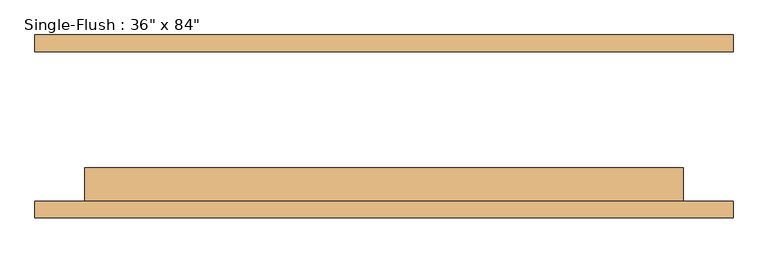
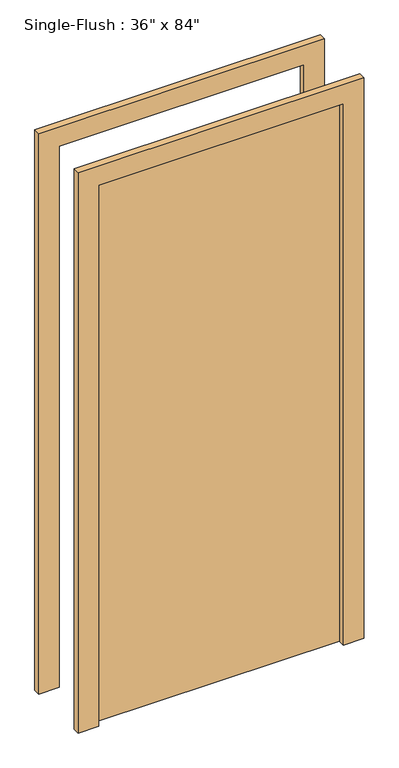
"""IFC4 building model written with IfcOpenShell, lengths in millimetres: door geometry."""

from ifc_helpers import new_model, si_unit, frame, origin, origin_with_axes, place, context, project, spatial, polyline, outline, extrude, source, transform, mapped, element, save


def door_a90ba1ad(model_context):
    return source(origin(), model_context, "Body", "SweptSolid", [
        extrude(outline(polyline([(2209.8, -533.4), (0.0, -533.4), (0.0, -457.2), (2133.6, -457.2), (2133.6, 457.2), (0.0, 457.2), (0.0, 533.4), (2209.8, 533.4), (2209.8, -533.4)])), frame((0.0, -139.7, 0.0), z_axis=(0.0, 1.0, 0.0), x_axis=(0.0, 0.0, 1.0)), (0.0, 0.0, 1.0), 25.4),
        extrude(outline(polyline([(2209.8, 533.4), (2209.8, -533.4), (0.0, -533.4), (0.0, -457.2), (2133.6, -457.2), (2133.6, 457.2), (0.0, 457.2), (0.0, 533.4), (2209.8, 533.4)])), frame((0.0, 114.3, 0.0), z_axis=(0.0, 1.0, 0.0), x_axis=(0.0, 0.0, 1.0)), (0.0, 0.0, 1.0), 25.4),
        extrude(outline(polyline([(457.2, -63.5), (457.2, -114.3), (-457.2, -114.3), (-457.2, -63.5), (457.2, -63.5)])), origin_with_axes(), (0.0, 0.0, 1.0), 2133.6),
    ])


if __name__ == "__main__":
    model = new_model("IFC4")
    model_context = context("Model", 3, world=origin())
    ifc_project = project(units=[si_unit("LENGTHUNIT", "METRE", prefix="MILLI")], contexts=[model_context])
    site = spatial("IfcSite", under=ifc_project)
    building = spatial("IfcBuilding", under=site)
    placement = place(None, origin())
    door_shape = door_a90ba1ad(model_context)
    element("IfcDoor", 1, ObjectType="Single-Flush : 36\" x 84\"", at=placement, inside=building, context=model_context, shape_type="MappedRepresentation", body=[
        mapped(door_shape, transform((0.0, 0.0, 0.0), x_axis=(1.0, 0.0, 0.0), y_axis=(0.0, 1.0, 0.0), z_axis=(0.0, 0.0, 1.0))),
    ])
    save(model, "model.ifc")

# Revit data of these elements
# Type "Single-Flush : 36\" x 84\""
#   Type Mark = "1"
#   Assembly Code = "C1020"
#   Thickness = 0' - 2"
#   Height = 7' - 0"
#   Trim Projection Ext = 0' - 1"
#   Trim Projection Int = 0' - 1"
#   Trim Width = 0' - 3"
#   Width = 3' - 0"
#   Door Material = Door - Panel
#   Frame Material = Door - Frame
#   Function = (empty or 0)
#   Wall Closure = (empty or 0)
# Element 1 (IfcDoor, "Single-Flush : 36\" x 84\"")
#   Materials on its faces: "Door - Frame", "Door - Panel"
# Materials
#   "Door - Panel": class "Wood", colour RGB 114 82 51, transparency 0
#   "Door - Frame": colour RGB 153 76 43, transparency 0
